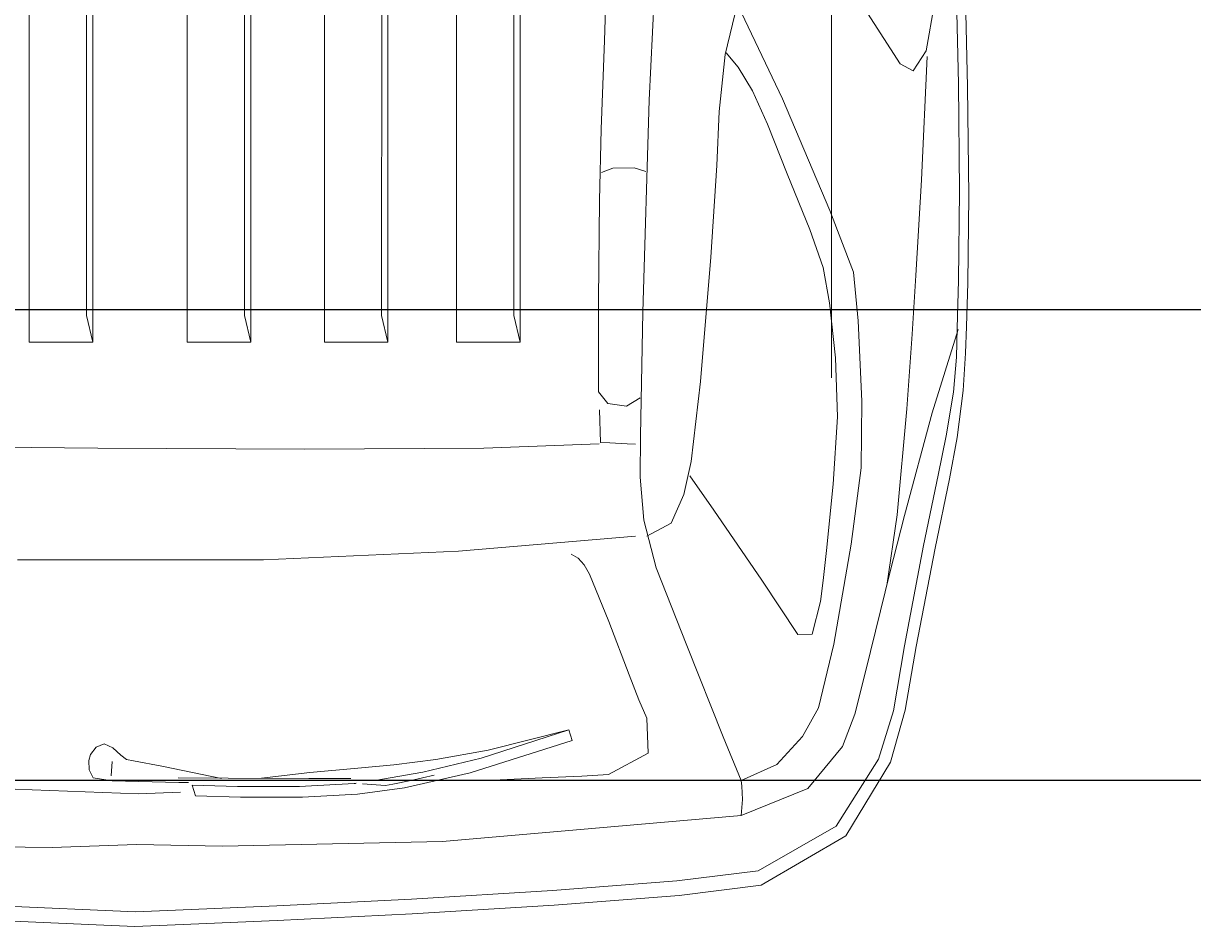
# Model space of a CAD drawing. Units: inches. Extents: x -5 to 482, y -460 to 66.
# Tile 5 of 31: x 66 to 91, y -389 to -370. Entities that reach past the tile are written whole.
import ezdxf

# ---------------------------------------------------------------- set-up
doc = ezdxf.new("R2010")
doc.units = ezdxf.units.IN
doc.header["$MEASUREMENT"] = 0
doc.layers.add('A-ANNO-DIMS', color=2, linetype='Continuous', lineweight=18)
doc.layers.add('A-EQPM-VEHI', color=8, linetype='Continuous', lineweight=13)
doc.styles.get("Standard").update_dxf_attribs({"font": 'arial.ttf'})
doc.dimstyles.get("Standard").update_dxf_attribs({"dimtxt": 0.18, "dimasz": 0.18, "dimexe": 0.18, "dimexo": 0.0625, "dimgap": 0.09, "dimtad": 0, "dimtih": 1, "dimtoh": 1, "dimdec": 0, "dimzin": 0, "dimdsep": 46, "dimlunit": 3, "dimtxsty": 'Standard', "dimcen": 0.09, "dimadec": 0, "dimazin": 0, "dimtfac": 1, "dimtdec": 0, "dimtofl": 0, "dimtmove": 0, "dimatfit": 3, "dimfxl": 1, "dimtolj": 1, "dimtzin": 0, "dimarcsym": 0})

# ---------------------------------------------------------------- blocks, each defined once
blk = doc.blocks.new('*D72')
at = {"layer": 'A-ANNO-DIMS', "color": 0, "lineweight": -2, "transparency": 16777216}
for p, q in [((144.314, -375.861), (-4.903, -375.861)), ((-4.723, -376.041), (-4.723, -380.679)), ((-4.723, -385.681), (-4.723, -381.043)), ((144.314, -385.861), (-4.903, -385.861))]:
    blk.add_line(p, q, dxfattribs=at)
at = {"layer": 'A-ANNO-DIMS', "color": 0, "transparency": 16777216}
for points in [[(-4.753, -376.041), (-4.693, -376.041), (-4.723, -375.861)], [(-4.753, -385.681), (-4.693, -385.681), (-4.723, -385.861)]]:
    blk.add_solid(points, dxfattribs=at)
at = {"layer": 'Defpoints', "color": 0, "transparency": 16777216}
for p in [(144.377, -375.861), (-4.723, -385.861), (144.377, -385.861)]:
    blk.add_point(p, dxfattribs=at)
at = {"layer": 'A-ANNO-DIMS', "color": 0, "transparency": 16777216, "insert": (-4.723, -380.861), "char_height": 0.18, "attachment_point": 5}
blk.add_mtext('\\A1;0\'-10"', dxfattribs=at)

msp = doc.modelspace()

# ---------------------------------------------------------------- linework, layer by layer
at = {"layer": 'A-EQPM-VEHI'}
for p, q in [((66.616, -376.546), (66.616, -341.062)), ((67.833, -375.982), (67.845, -341.174)), ((67.967, -341.062), (67.967, -376.546)), ((67.968, -341.062), (67.968, -376.546)), ((69.977, -376.546), (69.977, -341.062)), ((71.194, -375.982), (71.207, -341.174)), ((71.329, -341.062), (71.329, -376.546)), ((71.33, -341.062), (71.33, -376.546)), ((72.891, -376.546), (72.891, -341.062)), ((74.108, -375.982), (74.121, -341.174)), ((74.242, -341.062), (74.242, -376.546)), ((74.243, -341.062), (74.243, -376.546)), ((75.7, -376.546), (75.7, -341.062)), ((76.918, -375.982), (76.932, -341.174)), ((77.053, -341.062), (77.053, -376.546)), ((83.675, -365.165), (83.675, -377.301)), ((78.844, -370.135), (78.965, -366.416)), ((79.982, -367.491), (79.796, -371.406)), ((83.578, -368.208), (85.131, -370.632)), ((81.671, -369.349), (81.415, -370.43)), ((81.57, -369.146), (82.633, -371.377)), ((85.682, -370.358), (85.862, -369.35)), ((86.369, -371.057), (86.325, -369.124)), ((86.521, -369.111), (86.566, -371.117)), ((78.775, -372.018), (78.844, -370.135)), ((81.415, -370.43), (81.286, -371.646)), ((81.435, -370.396), (81.685, -370.7)), ((85.408, -370.779), (85.682, -370.358)), ((85.703, -370.476), (85.584, -373.094)), ((81.685, -370.7), (81.995, -371.207)), ((85.131, -370.632), (85.408, -370.779)), ((86.392, -373.338), (86.369, -371.057)), ((81.995, -371.207), (82.313, -371.916)), ((86.566, -371.117), (86.591, -373.437)), ((79.796, -371.406), (79.662, -375.907)), ((82.633, -371.377), (83.637, -373.751)), ((81.286, -371.646), (81.232, -372.795)), ((78.737, -373.534), (78.775, -372.018)), ((82.313, -371.916), (82.732, -372.967)), ((81.232, -372.795), (81.107, -374.739)), ((79.024, -372.847), (78.782, -372.941)), ((79.479, -372.843), (79.024, -372.847)), ((79.725, -372.922), (79.479, -372.843)), ((82.732, -372.967), (83.211, -374.154)), ((85.584, -373.094), (85.462, -375.132)), ((78.72, -375.649), (78.737, -373.534)), ((86.375, -375.235), (86.392, -373.338)), ((86.591, -373.437), (86.573, -375.287)), ((83.637, -373.751), (84.137, -375.058)), ((83.211, -374.154), (83.495, -374.957)), ((81.107, -374.739), (80.884, -377.382)), ((83.495, -374.957), (83.627, -375.713)), ((84.137, -375.058), (84.241, -376.091)), ((85.462, -375.132), (85.387, -376.376)), ((86.344, -376.249), (86.375, -375.235)), ((86.573, -375.287), (86.541, -376.214)), ((78.719, -377.601), (78.72, -375.649)), ((83.627, -375.713), (83.758, -376.881)), ((67.967, -376.546), (67.833, -375.982)), ((71.329, -376.546), (71.194, -375.982)), ((74.242, -376.546), (74.108, -375.982)), ((77.053, -376.546), (76.918, -375.982)), ((79.662, -375.907), (79.61, -378.538)), ((84.241, -376.091), (84.315, -377.799)), ((86.367, -376.274), (85.81, -378.05)), ((86.327, -376.863), (86.344, -376.249)), ((86.541, -376.214), (86.523, -376.781)), ((67.968, -376.546), (66.616, -376.546)), ((71.33, -376.546), (69.977, -376.546)), ((74.243, -376.546), (72.891, -376.546)), ((77.053, -376.546), (75.7, -376.546)), ((85.387, -376.376), (85.277, -377.962)), ((86.523, -376.781), (86.473, -377.576)), ((83.758, -376.881), (83.8, -378.133)), ((86.263, -377.607), (86.327, -376.863)), ((80.884, -377.382), (80.691, -379.079)), ((78.919, -377.85), (78.719, -377.601)), ((79.606, -377.731), (79.316, -377.906)), ((84.315, -377.799), (84.306, -379.214)), ((86.112, -378.536), (86.263, -377.607)), ((86.473, -377.576), (86.346, -378.571)), ((78.739, -377.985), (78.761, -378.678)), ((79.316, -377.906), (78.919, -377.85)), ((85.277, -377.962), (85.07, -380.217)), ((85.81, -378.05), (85.223, -380.231)), ((83.8, -378.133), (83.706, -379.56)), ((79.61, -378.538), (79.608, -379.415)), ((85.937, -379.373), (86.112, -378.536)), ((68.079, -378.796), (63.876, -378.752)), ((72.473, -378.82), (68.079, -378.796)), ((76.282, -378.798), (72.473, -378.82)), ((78.732, -378.707), (76.282, -378.798)), ((78.761, -378.678), (78.962, -378.687)), ((78.962, -378.687), (79.327, -378.703)), ((79.327, -378.703), (79.504, -378.712)), ((86.346, -378.571), (86.181, -379.453)), ((80.691, -379.079), (80.536, -379.783)), ((84.306, -379.214), (84.092, -380.837)), ((79.608, -379.415), (79.68, -380.33)), ((81.171, -380.116), (80.658, -379.383)), ((85.631, -380.868), (85.937, -379.373)), ((86.181, -379.453), (85.877, -380.922)), ((80.536, -379.783), (80.261, -380.39)), ((83.706, -379.56), (83.567, -380.973)), ((82.194, -381.6), (81.171, -380.116)), ((85.07, -380.217), (84.847, -381.714)), ((85.223, -380.231), (84.914, -381.444)), ((79.68, -380.33), (79.948, -381.342)), ((80.261, -380.39), (79.745, -380.666)), ((79.509, -380.666), (75.741, -380.985)), ((75.741, -380.985), (71.598, -381.169)), ((83.567, -380.973), (83.495, -381.612)), ((84.092, -380.837), (83.721, -382.962)), ((85.226, -383), (85.631, -380.868)), ((85.877, -380.922), (85.475, -383.012)), ((69.002, -381.173), (66.371, -381.169)), ((71.598, -381.169), (69.002, -381.173)), ((78.137, -381.052), (78.285, -381.139)), ((78.285, -381.139), (78.417, -381.277)), ((78.417, -381.277), (78.529, -381.477)), ((78.529, -381.477), (78.936, -382.484)), ((79.948, -381.342), (80.595, -382.994)), ((84.914, -381.444), (84.714, -382.253)), ((82.955, -382.761), (82.194, -381.6)), ((83.495, -381.612), (83.438, -382.053)), ((83.438, -382.053), (83.26, -382.749)), ((84.714, -382.253), (84.394, -383.551)), ((78.936, -382.484), (79.373, -383.612)), ((83.26, -382.749), (82.955, -382.761)), ((80.595, -382.994), (81.372, -384.931)), ((83.721, -382.962), (83.394, -384.315)), ((84.987, -384.381), (85.226, -383)), ((85.475, -383.012), (85.238, -384.368)), ((79.373, -383.612), (79.577, -384.146)), ((84.394, -383.551), (84.171, -384.45)), ((79.577, -384.146), (79.748, -384.535)), ((83.394, -384.315), (83.058, -384.926)), ((84.171, -384.45), (83.906, -385.136)), ((84.675, -385.408), (84.987, -384.381)), ((85.238, -384.368), (84.927, -385.47)), ((79.748, -384.535), (79.777, -385.277)), ((75.992, -385.698), (78.159, -385.009)), ((78.091, -384.784), (76.227, -385.385)), ((78.091, -384.784), (76.376, -385.214)), ((78.159, -385.009), (78.091, -384.784)), ((81.372, -384.931), (81.749, -385.862)), ((83.058, -384.926), (82.513, -385.521)), ((67.918, -385.304), (68.039, -385.152)), ((68.039, -385.152), (68.208, -385.084)), ((68.208, -385.084), (68.394, -385.169)), ((68.394, -385.169), (68.562, -385.321)), ((76.376, -385.214), (75.263, -385.416)), ((83.906, -385.136), (83.169, -386.031)), ((67.883, -385.435), (67.918, -385.304)), ((67.889, -385.632), (67.883, -385.435)), ((68.357, -385.758), (68.378, -385.453)), ((68.562, -385.321), (68.685, -385.414)), ((68.834, -385.44), (68.685, -385.414)), ((69.433, -385.555), (68.834, -385.44)), ((75.263, -385.416), (74.365, -385.525)), ((76.227, -385.385), (74.987, -385.682)), ((79.777, -385.277), (78.935, -385.734)), ((83.77, -386.831), (84.675, -385.408)), ((84.927, -385.47), (83.98, -387.036)), ((67.976, -385.805), (67.889, -385.632)), ((70.704, -385.814), (69.433, -385.555)), ((72.583, -385.692), (71.556, -385.811)), ((73.604, -385.599), (72.583, -385.692)), ((74.365, -385.525), (73.604, -385.599)), ((74.987, -385.682), (73.963, -385.86)), ((74.594, -386.014), (75.992, -385.698)), ((75.227, -385.744), (74.731, -385.86)), ((78.935, -385.734), (78.365, -385.766)), ((82.513, -385.521), (81.749, -385.862)), ((66.68, -386.057), (62.203, -385.884)), ((68.381, -385.867), (67.976, -385.805)), ((69.799, -385.902), (68.381, -385.867)), ((70.844, -385.811), (69.786, -385.806)), ((70, -385.904), (69.799, -385.902)), ((71.042, -385.989), (70.083, -385.96)), ((70.083, -385.96), (70.151, -386.184)), ((72.559, -385.816), (70.844, -385.811)), ((72.361, -385.989), (71.042, -385.989)), ((73.528, -385.925), (72.361, -385.989)), ((73.457, -385.817), (72.559, -385.816)), ((73.541, -385.923), (73.528, -385.925)), ((73.554, -385.921), (73.541, -385.923)), ((73.568, -385.92), (73.554, -385.921)), ((74.194, -385.967), (73.701, -385.93)), ((74.348, -385.938), (74.194, -385.967)), ((74.731, -385.86), (74.348, -385.938)), ((77.523, -385.806), (76.478, -385.851)), ((78.365, -385.766), (77.523, -385.806)), ((81.749, -385.862), (81.764, -385.98)), ((81.764, -385.98), (81.779, -386.263)), ((68.934, -386.14), (66.68, -386.057)), ((69.834, -386.107), (68.934, -386.14)), ((70.151, -386.184), (71.111, -386.213)), ((71.111, -386.213), (72.429, -386.214)), ((72.429, -386.214), (73.596, -386.149)), ((73.596, -386.149), (74.594, -386.014)), ((83.169, -386.031), (81.749, -386.606)), ((81.779, -386.263), (81.749, -386.606)), ((81.749, -386.606), (75.4, -387.155)), ((82.113, -387.777), (83.77, -386.831)), ((67.108, -387.283), (62.484, -387.232)), ((68.901, -387.22), (67.108, -387.283)), ((70.723, -387.256), (68.901, -387.22)), ((75.4, -387.155), (70.723, -387.256)), ((83.98, -387.036), (82.175, -388.083)), ((77.743, -388.198), (80.383, -387.994)), ((80.383, -387.994), (82.113, -387.777)), ((74.741, -388.378), (77.743, -388.198)), ((82.175, -388.083), (80.434, -388.302)), ((71.882, -388.522), (74.741, -388.378)), ((80.434, -388.302), (77.778, -388.508)), ((65.973, -388.525), (68.873, -388.652)), ((68.873, -388.652), (69.726, -388.618)), ((69.726, -388.618), (71.882, -388.522)), ((74.758, -388.69), (71.89, -388.834)), ((77.778, -388.508), (74.758, -388.69)), ((68.039, -388.93), (65.94, -388.834)), ((68.861, -388.964), (68.039, -388.93)), ((69.72, -388.93), (68.861, -388.964)), ((71.89, -388.834), (69.72, -388.93))]:
    msp.add_line(p, q, dxfattribs=at)

# ---------------------------------------------------------------- dimensions: what is measured, and where the dimension line sits
at = {"layer": 'A-ANNO-DIMS'}
dim = msp.add_linear_dim(base=(-4.723, -385.861), p1=(144.377, -375.861), p2=(144.377, -385.861), angle=90, dimstyle='Standard', override={"dimdec": 1, "dimlfac": 1, "dimrnd": 0, "dimzin": 1, "dimdsep": 46, "dimlunit": 4, "dimfrac": 2}, dxfattribs=at)
dim.commit()
dim.dimension.update_dxf_attribs({"geometry": '*D72', "text_midpoint": (-4.723, -380.861)})

doc.saveas('drawing.dxf')
